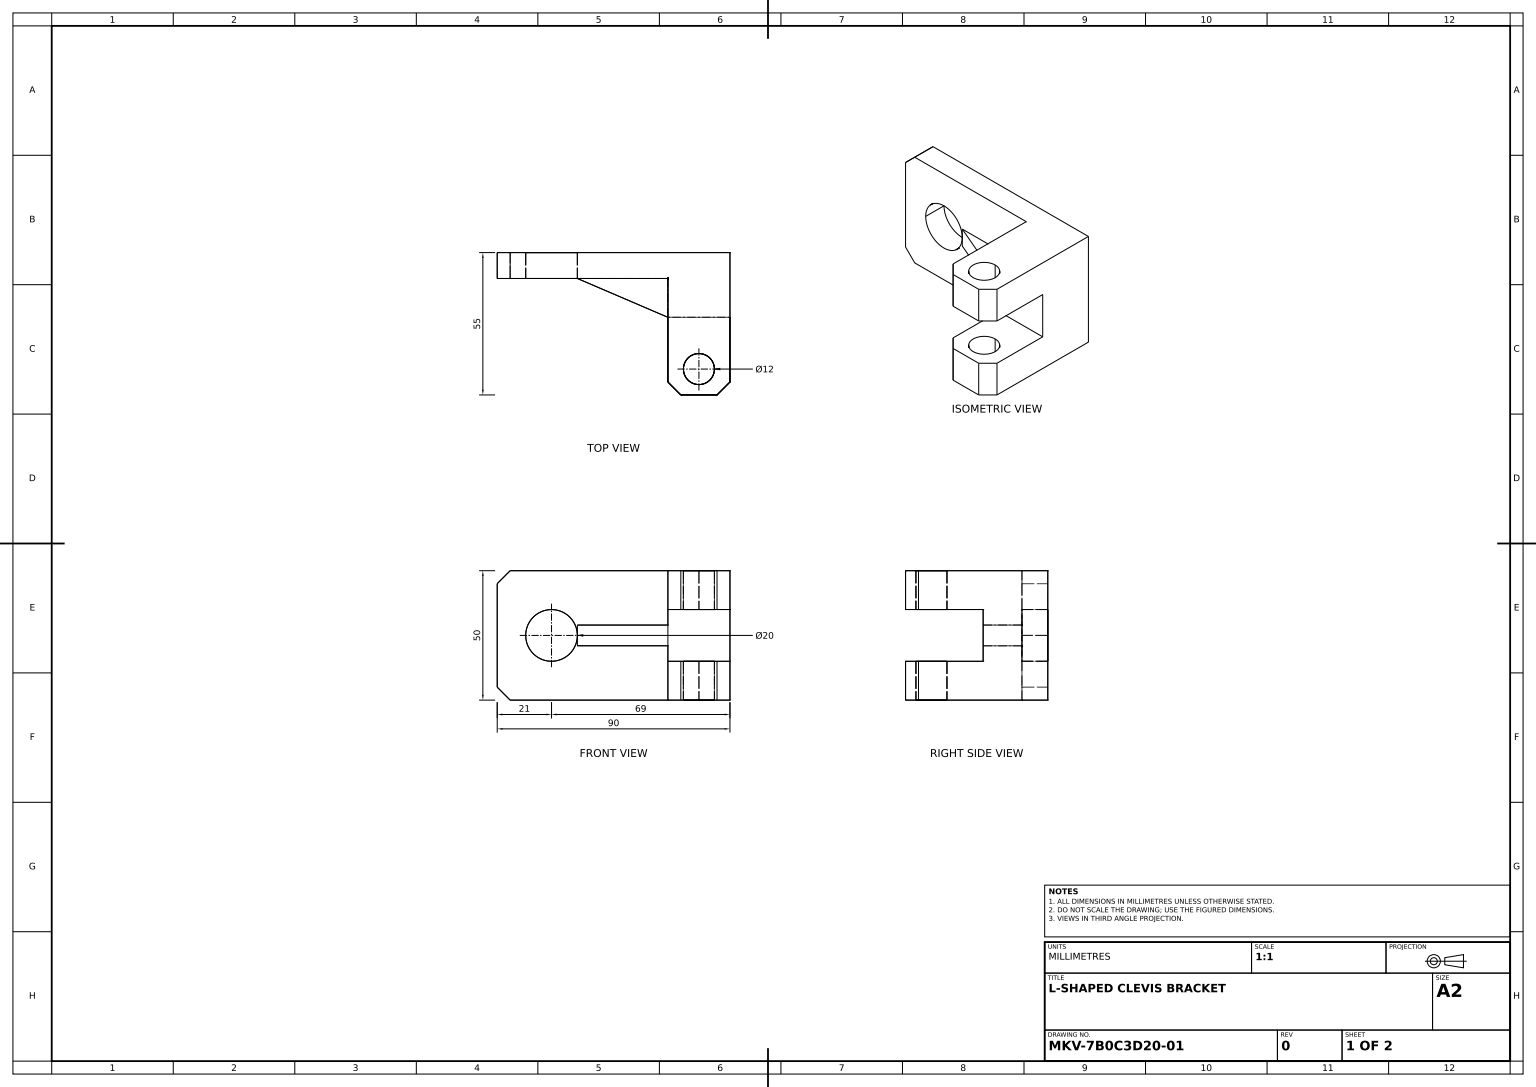
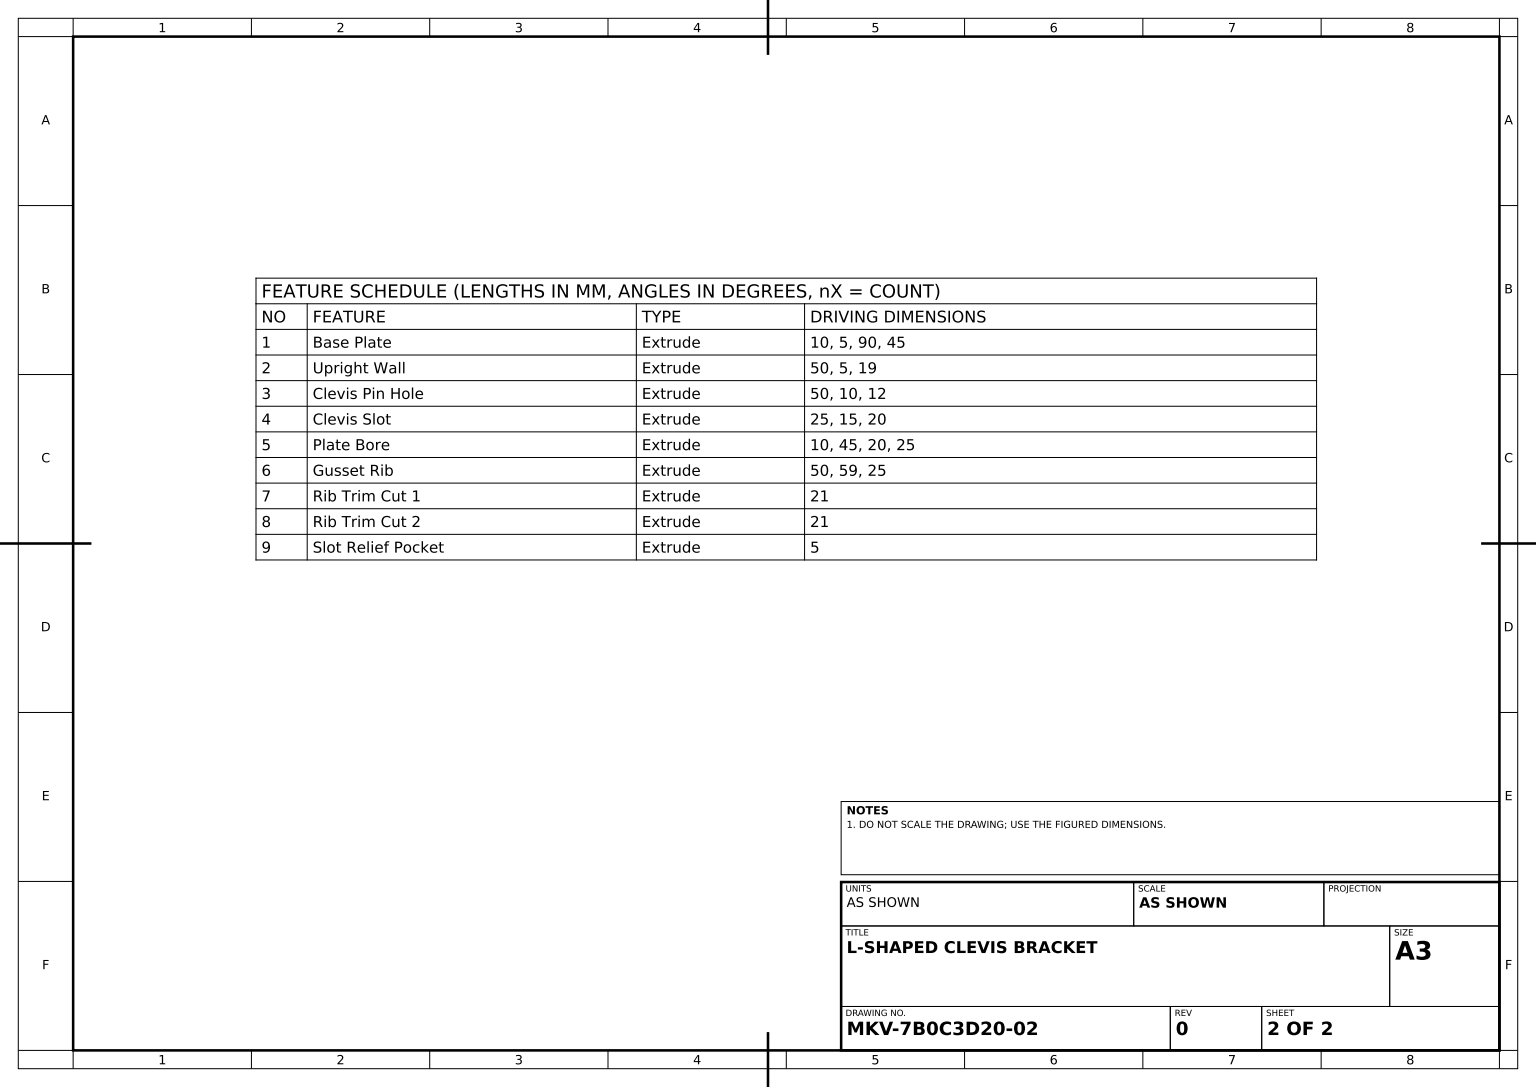
from build123d import *

# Parameters (mm, degrees)
BASE_PLATE_DEPTH            = 10
UPRIGHT_WALL_DEPTH          = 50
CLEVIS_PIN_HOLE_SKETCH_R    = 6
CLEVIS_PIN_HOLE_DEPTH       = 50
CLEVIS_SLOT_SKETCH_W        = 24
CLEVIS_SLOT_SKETCH_H        = 20
CLEVIS_SLOT_DEPTH           = 25
PLATE_BORE_SKETCH_R         = 10
PLATE_BORE_DEPTH            = 10
GUSSET_RIB_DEPTH            = 50
RIB_TRIM_CUT_1_DEPTH        = 21
RIB_TRIM_CUT_2_DEPTH        = 21
SLOT_RELIEF_POCKET_SKETCH_W = 24
SLOT_RELIEF_POCKET_SKETCH_H = 20
SLOT_RELIEF_POCKET_DEPTH    = 5


with BuildPart() as part:
    # Base Plate Profile → Base Plate (new body)
    with BuildSketch(Plane.XY):
        Polygon((90, 0), (5, 0), (0, 5), (0, 45), (5, 50), (90, 50), align=None)
    extrude(amount=BASE_PLATE_DEPTH)

    # Upright Wall Profile → Upright Wall (add)
    with BuildSketch(Plane.XZ):
        Polygon((90, 10), (90, 50), (85, 55), (71, 55), (66, 50), (66, 10), align=None)
    extrude(amount=-UPRIGHT_WALL_DEPTH)

    # Clevis Pin Hole Sketch → Clevis Pin Hole (cut)
    with BuildSketch(Plane.XZ):
        with Locations(Location((78, 45, 0), (0, 0, 270))):
            Circle(CLEVIS_PIN_HOLE_SKETCH_R)
    extrude(amount=-CLEVIS_PIN_HOLE_DEPTH, mode=Mode.SUBTRACT)

    # Clevis Slot Sketch → Clevis Slot (cut)
    with BuildSketch(Plane.XY.offset(55)):
        with Locations((78, 25)):
            Rectangle(CLEVIS_SLOT_SKETCH_W, CLEVIS_SLOT_SKETCH_H)
    extrude(amount=-CLEVIS_SLOT_DEPTH, mode=Mode.SUBTRACT)

    # Plate Bore Sketch → Plate Bore (cut)
    with BuildSketch(Plane.XY.offset(10)):
        with Locations((21, 25)):
            Circle(PLATE_BORE_SKETCH_R)
    extrude(amount=-PLATE_BORE_DEPTH, mode=Mode.SUBTRACT)

    # Gusset Rib Profile → Gusset Rib (add)
    with BuildSketch(Plane.XZ):
        Polygon((66, 10), (66, 25), (31, 10), align=None)
    extrude(amount=-GUSSET_RIB_DEPTH)

    # Rib Trim Cut 1 Sketch → Rib Trim Cut 1 (cut)
    with BuildSketch(Plane.XZ):
        Polygon((66, 25), (66, 10), (31, 10), align=None)
    extrude(amount=-RIB_TRIM_CUT_1_DEPTH, mode=Mode.SUBTRACT)

    # Rib Trim Cut 2 Sketch → Rib Trim Cut 2 (cut)
    with BuildSketch(Plane(origin=(0, 50, 0), x_dir=(1, 0, 0), z_dir=(0, 1, 0))):
        Polygon((66, -25), (66, -10), (31, -10), align=None)
    extrude(amount=-RIB_TRIM_CUT_2_DEPTH, mode=Mode.SUBTRACT)

    # Slot Relief Pocket Sketch → Slot Relief Pocket (cut)
    with BuildSketch(Plane.XY.offset(30)):
        with Locations((78, 25)):
            Rectangle(SLOT_RELIEF_POCKET_SKETCH_W, SLOT_RELIEF_POCKET_SKETCH_H)
    extrude(amount=-SLOT_RELIEF_POCKET_DEPTH, mode=Mode.SUBTRACT)


solid = part.part
